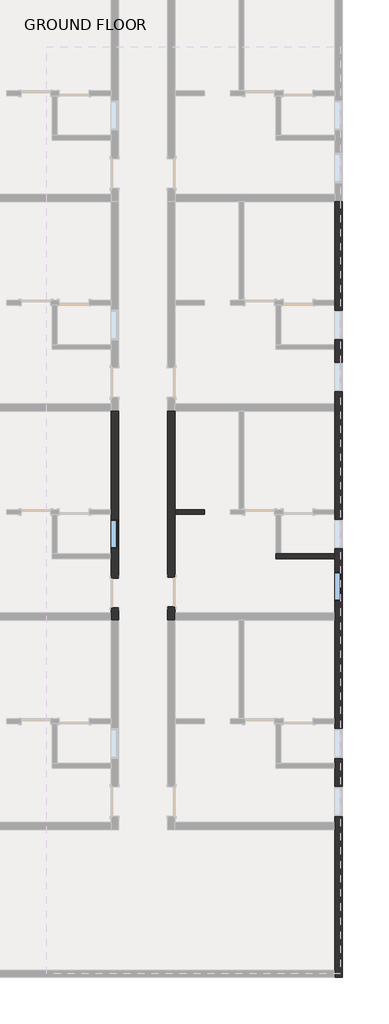
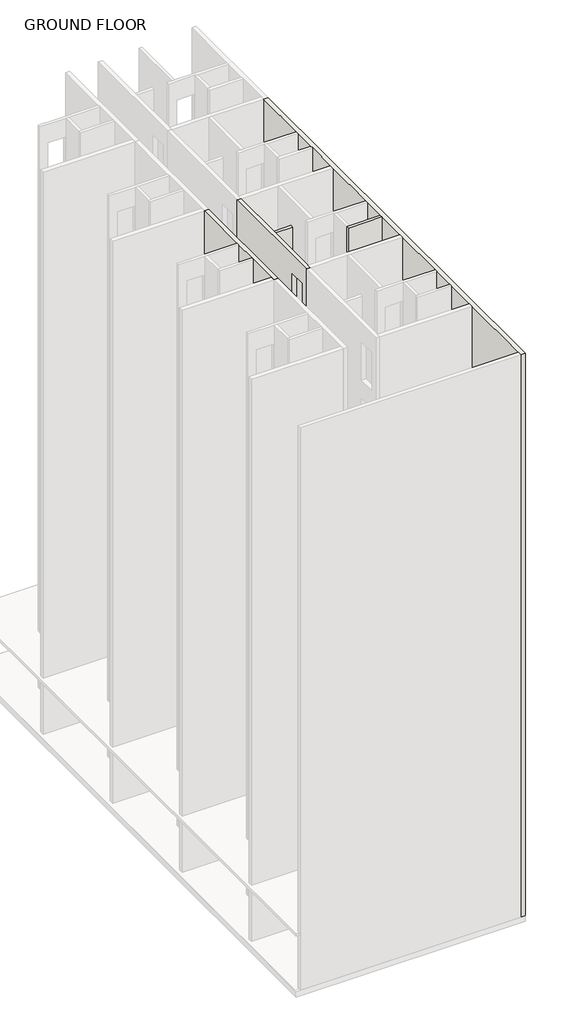
# One storey, part 4 of 7: 5 walls, 2 windows.
"""IFC4 building model written with IfcOpenShell, lengths in millimetres."""

from ifc_helpers import new_model, si_unit, origin, origin_with_axes, place, context, project, spatial, polyline, outline, extrude, faceted_brep, transform, mapped, element, save
from components import window_c1f32544

model = new_model("IFC4")

# Units and contexts
model_context = context("Model", 3, world=origin())
ifc_project = project(units=[si_unit("LENGTHUNIT", "METRE", prefix="MILLI")], contexts=[model_context])

# Site, building, storey
site = spatial("IfcSite", under=ifc_project)
building = spatial("IfcBuilding", under=site)
storey = spatial("IfcBuildingStorey", under=building, Name="GROUND FLOOR", Elevation=0.0)

# Walls
placement = place(None, origin())
element("IfcWall", 1, ObjectType="Generic - 8\"", at=placement, inside=storey, context=model_context, shape_type="Brep", body=[
    faceted_brep([(-5558.2902461, -4354.5289408, 0.0), (-5558.2902461, -4125.9289408, 0.0), (-5558.2902461, -3935.4289408, 0.0), (-5558.2902461, -3935.4289408, 2133.6), (-5558.2902461, -3021.0289408, 2133.6), (-5558.2902461, -3021.0289408, 0.0), (-5558.2902461, -1077.9289408, 0.0), (-5558.2902461, -925.5289408, 0.0), (-5558.2902461, 2122.4710592, 0.0), (-5558.2902461, 2122.4710592, 32004.0), (-5558.2902461, -925.5289408, 32004.0), (-5558.2902461, -1077.9289408, 32004.0), (-5558.2902461, -4125.9289408, 32004.0), (-5558.2902461, -4354.5289408, 32004.0), (-5558.2902461, -3021.0289408, 3200.4), (-5558.2902461, -3935.4289408, 3200.4), (-5558.2902461, -3935.4289408, 5334.0), (-5558.2902461, -3021.0289408, 5334.0), (-5558.2902461, -3021.0289408, 6400.8), (-5558.2902461, -3935.4289408, 6400.8), (-5558.2902461, -3935.4289408, 8534.4), (-5558.2902461, -3021.0289408, 8534.4), (-5558.2902461, -3021.0289408, 9601.2), (-5558.2902461, -3935.4289408, 9601.2), (-5558.2902461, -3935.4289408, 11734.8), (-5558.2902461, -3021.0289408, 11734.8), (-5558.2902461, -3021.0289408, 12801.6), (-5558.2902461, -3935.4289408, 12801.6), (-5558.2902461, -3935.4289408, 14935.2), (-5558.2902461, -3021.0289408, 14935.2), (-5558.2902461, -3021.0289408, 16002.0), (-5558.2902461, -3935.4289408, 16002.0), (-5558.2902461, -3935.4289408, 18135.6), (-5558.2902461, -3021.0289408, 18135.6), (-5558.2902461, -3021.0289408, 19202.4), (-5558.2902461, -3935.4289408, 19202.4), (-5558.2902461, -3935.4289408, 21336.0), (-5558.2902461, -3021.0289408, 21336.0), (-5558.2902461, -3021.0289408, 22402.8), (-5558.2902461, -3935.4289408, 22402.8), (-5558.2902461, -3935.4289408, 24536.4), (-5558.2902461, -3021.0289408, 24536.4), (-5558.2902461, -3021.0289408, 25603.2), (-5558.2902461, -3935.4289408, 25603.2), (-5558.2902461, -3935.4289408, 27736.8), (-5558.2902461, -3021.0289408, 27736.8), (-5558.2902461, -3021.0289408, 28803.6), (-5558.2902461, -3935.4289408, 28803.6), (-5558.2902461, -3935.4289408, 30937.2), (-5558.2902461, -3021.0289408, 30937.2), (-5786.8902461, -3935.4289408, 2133.6), (-5786.8902461, -3935.4289408, 0.0), (-5786.8902461, -4354.5289408, 0.0), (-5786.8902461, -4354.5289408, 32004.0), (-5786.8902461, 2122.4710592, 32004.0), (-5786.8902461, 2122.4710592, 0.0), (-5786.8902461, -3021.0289408, 0.0), (-5786.8902461, -3021.0289408, 2133.6), (-5786.8902461, -3021.0289408, 3200.4), (-5786.8902461, -3021.0289408, 5334.0), (-5786.8902461, -3935.4289408, 5334.0), (-5786.8902461, -3935.4289408, 3200.4), (-5786.8902461, -3021.0289408, 6400.8), (-5786.8902461, -3021.0289408, 8534.4), (-5786.8902461, -3935.4289408, 8534.4), (-5786.8902461, -3935.4289408, 6400.8), (-5786.8902461, -3021.0289408, 9601.2), (-5786.8902461, -3021.0289408, 11734.8), (-5786.8902461, -3935.4289408, 11734.8), (-5786.8902461, -3935.4289408, 9601.2), (-5786.8902461, -3021.0289408, 12801.6), (-5786.8902461, -3021.0289408, 14935.2), (-5786.8902461, -3935.4289408, 14935.2), (-5786.8902461, -3935.4289408, 12801.6), (-5786.8902461, -3021.0289408, 16002.0), (-5786.8902461, -3021.0289408, 18135.6), (-5786.8902461, -3935.4289408, 18135.6), (-5786.8902461, -3935.4289408, 16002.0), (-5786.8902461, -3021.0289408, 19202.4), (-5786.8902461, -3021.0289408, 21336.0), (-5786.8902461, -3935.4289408, 21336.0), (-5786.8902461, -3935.4289408, 19202.4), (-5786.8902461, -3021.0289408, 22402.8), (-5786.8902461, -3021.0289408, 24536.4), (-5786.8902461, -3935.4289408, 24536.4), (-5786.8902461, -3935.4289408, 22402.8), (-5786.8902461, -3021.0289408, 25603.2), (-5786.8902461, -3021.0289408, 27736.8), (-5786.8902461, -3935.4289408, 27736.8), (-5786.8902461, -3935.4289408, 25603.2), (-5786.8902461, -3021.0289408, 28803.6), (-5786.8902461, -3021.0289408, 30937.2), (-5786.8902461, -3935.4289408, 30937.2), (-5786.8902461, -3935.4289408, 28803.6)], [[[0, 1, 2, 3, 4, 5, 6, 7, 8, 9, 10, 11, 12, 13], [14, 15, 16, 17], [18, 19, 20, 21], [22, 23, 24, 25], [26, 27, 28, 29], [30, 31, 32, 33], [34, 35, 36, 37], [38, 39, 40, 41], [42, 43, 44, 45], [46, 47, 48, 49]], [[50, 51, 52, 53, 54, 55, 56, 57], [58, 59, 60, 61], [62, 63, 64, 65], [66, 67, 68, 69], [70, 71, 72, 73], [74, 75, 76, 77], [78, 79, 80, 81], [82, 83, 84, 85], [86, 87, 88, 89], [90, 91, 92, 93]], [[56, 55, 8, 7, 6, 5]], [[52, 51, 2, 1, 0]], [[13, 12, 11, 10, 9, 54, 53]], [[0, 13, 53, 52]], [[9, 8, 55, 54]], [[3, 2, 51, 50]], [[4, 3, 50, 57]], [[5, 4, 57, 56]], [[15, 14, 58, 61]], [[16, 15, 61, 60]], [[17, 16, 60, 59]], [[14, 17, 59, 58]], [[19, 18, 62, 65]], [[20, 19, 65, 64]], [[21, 20, 64, 63]], [[18, 21, 63, 62]], [[23, 22, 66, 69]], [[24, 23, 69, 68]], [[25, 24, 68, 67]], [[22, 25, 67, 66]], [[27, 26, 70, 73]], [[28, 27, 73, 72]], [[29, 28, 72, 71]], [[26, 29, 71, 70]], [[31, 30, 74, 77]], [[32, 31, 77, 76]], [[33, 32, 76, 75]], [[30, 33, 75, 74]], [[35, 34, 78, 81]], [[36, 35, 81, 80]], [[37, 36, 80, 79]], [[34, 37, 79, 78]], [[39, 38, 82, 85]], [[40, 39, 85, 84]], [[41, 40, 84, 83]], [[38, 41, 83, 82]], [[43, 42, 86, 89]], [[44, 43, 89, 88]], [[45, 44, 88, 87]], [[42, 45, 87, 86]], [[47, 46, 90, 93]], [[48, 47, 93, 92]], [[49, 48, 92, 91]], [[46, 49, 91, 90]]]),
])
element("IfcWall", 2, ObjectType="INNER WALL 2", at=placement, inside=storey, context=model_context, shape_type="Brep", body=[
    faceted_brep([(-605.2902461, -2297.1289408, 0.0), (-2281.6902461, -2297.1289408, 0.0), (-2434.0902461, -2297.1289408, 0.0), (-2434.0902461, -2297.1289408, 32004.0), (-2281.6902461, -2297.1289408, 32004.0), (-605.2902461, -2297.1289408, 32004.0), (-605.2902461, -2449.5289408, 0.0), (-605.2902461, -2449.5289408, 32004.0), (-2434.0902461, -2449.5289408, 32004.0), (-2434.0902461, -2449.5289408, 0.0)], [[[0, 1, 2, 3, 4, 5]], [[6, 7, 8, 9]], [[2, 1, 0, 6, 9]], [[5, 4, 3, 8, 7]], [[3, 2, 9, 8]], [[0, 5, 7, 6]]]),
])
element("IfcWall", 3, ObjectType="INNER WALL 2", at=placement, inside=storey, context=model_context, shape_type="SweptSolid", body=[
    extrude(outline(polyline([(-4643.8902461, -1077.9289408), (-5558.2902461, -1077.9289408), (-5558.2902461, -925.5289408), (-4643.8902461, -925.5289408), (-4643.8902461, -1077.9289408)])), origin_with_axes(), (0.0, 0.0, 1.0), 32004.0),
])
element("IfcWall", 4, ObjectType="OUTER WALL", at=placement, inside=storey, context=model_context, shape_type="Brep", body=[
    faceted_brep([(-376.6902461, -15403.5289408, 0.0), (-376.6902461, 8599.4710592, 0.0), (-376.6902461, 8599.4710592, 32004.0), (-376.6902461, -15403.5289408, 32004.0), (-376.6902461, -10412.4289408, 2133.6), (-376.6902461, -9498.0289408, 2133.6), (-376.6902461, -9498.0289408, 914.4), (-376.6902461, -10412.4289408, 914.4), (-376.6902461, -8621.7289408, 2133.6), (-376.6902461, -7707.3289408, 2133.6), (-376.6902461, -7707.3289408, 914.4), (-376.6902461, -8621.7289408, 914.4), (-376.6902461, -3763.9789408, 2133.6), (-376.6902461, -2849.5789408, 2133.6), (-376.6902461, -2849.5789408, 914.4), (-376.6902461, -3763.9789408, 914.4), (-376.6902461, -2144.7289408, 2133.6), (-376.6902461, -1230.3289408, 2133.6), (-376.6902461, -1230.3289408, 914.4), (-376.6902461, -2144.7289408, 914.4), (-376.6902461, 2713.0210592, 2133.6), (-376.6902461, 3627.4210592, 2133.6), (-376.6902461, 3627.4210592, 914.4), (-376.6902461, 2713.0210592, 914.4), (-376.6902461, 4332.2710592, 2133.6), (-376.6902461, 5246.6710592, 2133.6), (-376.6902461, 5246.6710592, 914.4), (-376.6902461, 4332.2710592, 914.4), (-376.6902461, 4332.2710592, 5334.0), (-376.6902461, 5246.6710592, 5334.0), (-376.6902461, 5246.6710592, 4114.8), (-376.6902461, 4332.2710592, 4114.8), (-376.6902461, 2713.0210592, 5334.0), (-376.6902461, 3627.4210592, 5334.0), (-376.6902461, 3627.4210592, 4114.8), (-376.6902461, 2713.0210592, 4114.8), (-376.6902461, -2144.7289408, 5334.0), (-376.6902461, -1230.3289408, 5334.0), (-376.6902461, -1230.3289408, 4114.8), (-376.6902461, -2144.7289408, 4114.8), (-376.6902461, -3763.9789408, 5334.0), (-376.6902461, -2849.5789408, 5334.0), (-376.6902461, -2849.5789408, 4114.8), (-376.6902461, -3763.9789408, 4114.8), (-376.6902461, -8621.7289408, 5334.0), (-376.6902461, -7707.3289408, 5334.0), (-376.6902461, -7707.3289408, 4114.8), (-376.6902461, -8621.7289408, 4114.8), (-376.6902461, -10412.4289408, 5334.0), (-376.6902461, -9498.0289408, 5334.0), (-376.6902461, -9498.0289408, 4114.8), (-376.6902461, -10412.4289408, 4114.8), (-376.6902461, 4332.2710592, 8534.4), (-376.6902461, 5246.6710592, 8534.4), (-376.6902461, 5246.6710592, 7315.2), (-376.6902461, 4332.2710592, 7315.2), (-376.6902461, 2713.0210592, 8534.4), (-376.6902461, 3627.4210592, 8534.4), (-376.6902461, 3627.4210592, 7315.2), (-376.6902461, 2713.0210592, 7315.2), (-376.6902461, -2144.7289408, 8534.4), (-376.6902461, -1230.3289408, 8534.4), (-376.6902461, -1230.3289408, 7315.2), (-376.6902461, -2144.7289408, 7315.2), (-376.6902461, -3763.9789408, 8534.4), (-376.6902461, -2849.5789408, 8534.4), (-376.6902461, -2849.5789408, 7315.2), (-376.6902461, -3763.9789408, 7315.2), (-376.6902461, -8621.7289408, 8534.4), (-376.6902461, -7707.3289408, 8534.4), (-376.6902461, -7707.3289408, 7315.2), (-376.6902461, -8621.7289408, 7315.2), (-376.6902461, -10412.4289408, 8534.4), (-376.6902461, -9498.0289408, 8534.4), (-376.6902461, -9498.0289408, 7315.2), (-376.6902461, -10412.4289408, 7315.2), (-376.6902461, 4332.2710592, 11734.8), (-376.6902461, 5246.6710592, 11734.8), (-376.6902461, 5246.6710592, 10515.6), (-376.6902461, 4332.2710592, 10515.6), (-376.6902461, 2713.0210592, 11734.8), (-376.6902461, 3627.4210592, 11734.8), (-376.6902461, 3627.4210592, 10515.6), (-376.6902461, 2713.0210592, 10515.6), (-376.6902461, -2144.7289408, 11734.8), (-376.6902461, -1230.3289408, 11734.8), (-376.6902461, -1230.3289408, 10515.6), (-376.6902461, -2144.7289408, 10515.6), (-376.6902461, -3763.9789408, 11734.8), (-376.6902461, -2849.5789408, 11734.8), (-376.6902461, -2849.5789408, 10515.6), (-376.6902461, -3763.9789408, 10515.6), (-376.6902461, -8621.7289408, 11734.8), (-376.6902461, -7707.3289408, 11734.8), (-376.6902461, -7707.3289408, 10515.6), (-376.6902461, -8621.7289408, 10515.6), (-376.6902461, -10412.4289408, 11734.8), (-376.6902461, -9498.0289408, 11734.8), (-376.6902461, -9498.0289408, 10515.6), (-376.6902461, -10412.4289408, 10515.6), (-376.6902461, 4332.2710592, 14935.2), (-376.6902461, 5246.6710592, 14935.2), (-376.6902461, 5246.6710592, 13716.0), (-376.6902461, 4332.2710592, 13716.0), (-376.6902461, 2713.0210592, 14935.2), (-376.6902461, 3627.4210592, 14935.2), (-376.6902461, 3627.4210592, 13716.0), (-376.6902461, 2713.0210592, 13716.0), (-376.6902461, -2144.7289408, 14935.2), (-376.6902461, -1230.3289408, 14935.2), (-376.6902461, -1230.3289408, 13716.0), (-376.6902461, -2144.7289408, 13716.0), (-376.6902461, -3763.9789408, 14935.2), (-376.6902461, -2849.5789408, 14935.2), (-376.6902461, -2849.5789408, 13716.0), (-376.6902461, -3763.9789408, 13716.0), (-376.6902461, -8621.7289408, 14935.2), (-376.6902461, -7707.3289408, 14935.2), (-376.6902461, -7707.3289408, 13716.0), (-376.6902461, -8621.7289408, 13716.0), (-376.6902461, -10412.4289408, 14935.2), (-376.6902461, -9498.0289408, 14935.2), (-376.6902461, -9498.0289408, 13716.0), (-376.6902461, -10412.4289408, 13716.0), (-376.6902461, 4332.2710592, 18135.6), (-376.6902461, 5246.6710592, 18135.6), (-376.6902461, 5246.6710592, 16916.4), (-376.6902461, 4332.2710592, 16916.4), (-376.6902461, 2713.0210592, 18135.6), (-376.6902461, 3627.4210592, 18135.6), (-376.6902461, 3627.4210592, 16916.4), (-376.6902461, 2713.0210592, 16916.4), (-376.6902461, -2144.7289408, 18135.6), (-376.6902461, -1230.3289408, 18135.6), (-376.6902461, -1230.3289408, 16916.4), (-376.6902461, -2144.7289408, 16916.4), (-376.6902461, -3763.9789408, 18135.6), (-376.6902461, -2849.5789408, 18135.6), (-376.6902461, -2849.5789408, 16916.4), (-376.6902461, -3763.9789408, 16916.4), (-376.6902461, -8621.7289408, 18135.6), (-376.6902461, -7707.3289408, 18135.6), (-376.6902461, -7707.3289408, 16916.4), (-376.6902461, -8621.7289408, 16916.4), (-376.6902461, -10412.4289408, 18135.6), (-376.6902461, -9498.0289408, 18135.6), (-376.6902461, -9498.0289408, 16916.4), (-376.6902461, -10412.4289408, 16916.4), (-376.6902461, 4332.2710592, 21336.0), (-376.6902461, 5246.6710592, 21336.0), (-376.6902461, 5246.6710592, 20116.8), (-376.6902461, 4332.2710592, 20116.8), (-376.6902461, 2713.0210592, 21336.0), (-376.6902461, 3627.4210592, 21336.0), (-376.6902461, 3627.4210592, 20116.8), (-376.6902461, 2713.0210592, 20116.8), (-376.6902461, -2144.7289408, 21336.0), (-376.6902461, -1230.3289408, 21336.0), (-376.6902461, -1230.3289408, 20116.8), (-376.6902461, -2144.7289408, 20116.8), (-376.6902461, -3763.9789408, 21336.0), (-376.6902461, -2849.5789408, 21336.0), (-376.6902461, -2849.5789408, 20116.8), (-376.6902461, -3763.9789408, 20116.8), (-376.6902461, -8621.7289408, 21336.0), (-376.6902461, -7707.3289408, 21336.0), (-376.6902461, -7707.3289408, 20116.8), (-376.6902461, -8621.7289408, 20116.8), (-376.6902461, -10412.4289408, 21336.0), (-376.6902461, -9498.0289408, 21336.0), (-376.6902461, -9498.0289408, 20116.8), (-376.6902461, -10412.4289408, 20116.8), (-376.6902461, 4332.2710592, 24536.4), (-376.6902461, 5246.6710592, 24536.4), (-376.6902461, 5246.6710592, 23317.2), (-376.6902461, 4332.2710592, 23317.2), (-376.6902461, 2713.0210592, 24536.4), (-376.6902461, 3627.4210592, 24536.4), (-376.6902461, 3627.4210592, 23317.2), (-376.6902461, 2713.0210592, 23317.2), (-376.6902461, -2144.7289408, 24536.4), (-376.6902461, -1230.3289408, 24536.4), (-376.6902461, -1230.3289408, 23317.2), (-376.6902461, -2144.7289408, 23317.2), (-376.6902461, -3763.9789408, 24536.4), (-376.6902461, -2849.5789408, 24536.4), (-376.6902461, -2849.5789408, 23317.2), (-376.6902461, -3763.9789408, 23317.2), (-376.6902461, -8621.7289408, 24536.4), (-376.6902461, -7707.3289408, 24536.4), (-376.6902461, -7707.3289408, 23317.2), (-376.6902461, -8621.7289408, 23317.2), (-376.6902461, -10412.4289408, 24536.4), (-376.6902461, -9498.0289408, 24536.4), (-376.6902461, -9498.0289408, 23317.2), (-376.6902461, -10412.4289408, 23317.2), (-376.6902461, 4332.2710592, 27736.8), (-376.6902461, 5246.6710592, 27736.8), (-376.6902461, 5246.6710592, 26517.6), (-376.6902461, 4332.2710592, 26517.6), (-376.6902461, -2144.7289408, 27736.8), (-376.6902461, -1230.3289408, 27736.8), (-376.6902461, -1230.3289408, 26517.6), (-376.6902461, -2144.7289408, 26517.6), (-376.6902461, -8621.7289408, 27736.8), (-376.6902461, -7707.3289408, 27736.8), (-376.6902461, -7707.3289408, 26517.6), (-376.6902461, -8621.7289408, 26517.6), (-376.6902461, -10412.4289408, 27736.8), (-376.6902461, -9498.0289408, 27736.8), (-376.6902461, -9498.0289408, 26517.6), (-376.6902461, -10412.4289408, 26517.6), (-376.6902461, -3763.9789408, 27736.8), (-376.6902461, -2849.5789408, 27736.8), (-376.6902461, -2849.5789408, 26517.6), (-376.6902461, -3763.9789408, 26517.6), (-376.6902461, 2713.0210592, 27736.8), (-376.6902461, 3627.4210592, 27736.8), (-376.6902461, 3627.4210592, 26517.6), (-376.6902461, 2713.0210592, 26517.6), (-376.6902461, 4332.2710592, 30937.2), (-376.6902461, 5246.6710592, 30937.2), (-376.6902461, 5246.6710592, 29718.0), (-376.6902461, 4332.2710592, 29718.0), (-376.6902461, 2713.0210592, 30937.2), (-376.6902461, 3627.4210592, 30937.2), (-376.6902461, 3627.4210592, 29718.0), (-376.6902461, 2713.0210592, 29718.0), (-376.6902461, -2144.7289408, 30937.2), (-376.6902461, -1230.3289408, 30937.2), (-376.6902461, -1230.3289408, 29718.0), (-376.6902461, -2144.7289408, 29718.0), (-376.6902461, -3763.9789408, 30937.2), (-376.6902461, -2849.5789408, 30937.2), (-376.6902461, -2849.5789408, 29718.0), (-376.6902461, -3763.9789408, 29718.0), (-376.6902461, -8621.7289408, 30937.2), (-376.6902461, -7707.3289408, 30937.2), (-376.6902461, -7707.3289408, 29718.0), (-376.6902461, -8621.7289408, 29718.0), (-376.6902461, -10412.4289408, 30937.2), (-376.6902461, -9498.0289408, 30937.2), (-376.6902461, -9498.0289408, 29718.0), (-376.6902461, -10412.4289408, 29718.0), (-605.2902461, -15403.5289408, 0.0), (-605.2902461, -15403.5289408, 32004.0), (-605.2902461, -15174.9289408, 32004.0), (-605.2902461, -10831.5289408, 32004.0), (-605.2902461, -10602.9289408, 32004.0), (-605.2902461, -8926.5289408, 32004.0), (-605.2902461, -8774.1289408, 32004.0), (-605.2902461, -7554.9289408, 32004.0), (-605.2902461, -7402.5289408, 32004.0), (-605.2902461, -4354.5289408, 32004.0), (-605.2902461, -4125.9289408, 32004.0), (-605.2902461, -2449.5289408, 32004.0), (-605.2902461, -2297.1289408, 32004.0), (-605.2902461, -1077.9289408, 32004.0), (-605.2902461, -925.5289408, 32004.0), (-605.2902461, 2122.4710592, 32004.0), (-605.2902461, 2351.0710592, 32004.0), (-605.2902461, 4027.4710592, 32004.0), (-605.2902461, 4179.8710592, 32004.0), (-605.2902461, 5399.0710592, 32004.0), (-605.2902461, 5551.4710592, 32004.0), (-605.2902461, 8599.4710592, 32004.0), (-605.2902461, 8599.4710592, 0.0), (-605.2902461, 5551.4710592, 0.0), (-605.2902461, 5399.0710592, 0.0), (-605.2902461, 4179.8710592, 0.0), (-605.2902461, 4027.4710592, 0.0), (-605.2902461, 2351.0710592, 0.0), (-605.2902461, 2122.4710592, 0.0), (-605.2902461, -925.5289408, 0.0), (-605.2902461, -1077.9289408, 0.0), (-605.2902461, -2297.1289408, 0.0), (-605.2902461, -2449.5289408, 0.0), (-605.2902461, -4125.9289408, 0.0), (-605.2902461, -4354.5289408, 0.0), (-605.2902461, -7402.5289408, 0.0), (-605.2902461, -7554.9289408, 0.0), (-605.2902461, -8774.1289408, 0.0), (-605.2902461, -8926.5289408, 0.0), (-605.2902461, -10602.9289408, 0.0), (-605.2902461, -10831.5289408, 0.0), (-605.2902461, -15174.9289408, 0.0), (-605.2902461, -10412.4289408, 2133.6), (-605.2902461, -10412.4289408, 914.4), (-605.2902461, -9498.0289408, 914.4), (-605.2902461, -9498.0289408, 2133.6), (-605.2902461, -8621.7289408, 2133.6), (-605.2902461, -8621.7289408, 914.4), (-605.2902461, -7707.3289408, 914.4), (-605.2902461, -7707.3289408, 2133.6), (-605.2902461, -3763.9789408, 2133.6), (-605.2902461, -3763.9789408, 914.4), (-605.2902461, -2849.5789408, 914.4), (-605.2902461, -2849.5789408, 2133.6), (-605.2902461, -2144.7289408, 2133.6), (-605.2902461, -2144.7289408, 914.4), (-605.2902461, -1230.3289408, 914.4), (-605.2902461, -1230.3289408, 2133.6), (-605.2902461, 2713.0210592, 2133.6), (-605.2902461, 2713.0210592, 914.4), (-605.2902461, 3627.4210592, 914.4), (-605.2902461, 3627.4210592, 2133.6), (-605.2902461, 4332.2710592, 2133.6), (-605.2902461, 4332.2710592, 914.4), (-605.2902461, 5246.6710592, 914.4), (-605.2902461, 5246.6710592, 2133.6), (-605.2902461, 4332.2710592, 5334.0), (-605.2902461, 4332.2710592, 4114.8), (-605.2902461, 5246.6710592, 4114.8), (-605.2902461, 5246.6710592, 5334.0), (-605.2902461, 2713.0210592, 5334.0), (-605.2902461, 2713.0210592, 4114.8), (-605.2902461, 3627.4210592, 4114.8), (-605.2902461, 3627.4210592, 5334.0), (-605.2902461, -2144.7289408, 5334.0), (-605.2902461, -2144.7289408, 4114.8), (-605.2902461, -1230.3289408, 4114.8), (-605.2902461, -1230.3289408, 5334.0), (-605.2902461, -3763.9789408, 5334.0), (-605.2902461, -3763.9789408, 4114.8), (-605.2902461, -2849.5789408, 4114.8), (-605.2902461, -2849.5789408, 5334.0), (-605.2902461, -8621.7289408, 5334.0), (-605.2902461, -8621.7289408, 4114.8), (-605.2902461, -7707.3289408, 4114.8), (-605.2902461, -7707.3289408, 5334.0), (-605.2902461, -10412.4289408, 5334.0), (-605.2902461, -10412.4289408, 4114.8), (-605.2902461, -9498.0289408, 4114.8), (-605.2902461, -9498.0289408, 5334.0), (-605.2902461, 4332.2710592, 8534.4), (-605.2902461, 4332.2710592, 7315.2), (-605.2902461, 5246.6710592, 7315.2), (-605.2902461, 5246.6710592, 8534.4), (-605.2902461, 2713.0210592, 8534.4), (-605.2902461, 2713.0210592, 7315.2), (-605.2902461, 3627.4210592, 7315.2), (-605.2902461, 3627.4210592, 8534.4), (-605.2902461, -2144.7289408, 8534.4), (-605.2902461, -2144.7289408, 7315.2), (-605.2902461, -1230.3289408, 7315.2), (-605.2902461, -1230.3289408, 8534.4), (-605.2902461, -3763.9789408, 8534.4), (-605.2902461, -3763.9789408, 7315.2), (-605.2902461, -2849.5789408, 7315.2), (-605.2902461, -2849.5789408, 8534.4), (-605.2902461, -8621.7289408, 8534.4), (-605.2902461, -8621.7289408, 7315.2), (-605.2902461, -7707.3289408, 7315.2), (-605.2902461, -7707.3289408, 8534.4), (-605.2902461, -10412.4289408, 8534.4), (-605.2902461, -10412.4289408, 7315.2), (-605.2902461, -9498.0289408, 7315.2), (-605.2902461, -9498.0289408, 8534.4), (-605.2902461, 4332.2710592, 11734.8), (-605.2902461, 4332.2710592, 10515.6), (-605.2902461, 5246.6710592, 10515.6), (-605.2902461, 5246.6710592, 11734.8), (-605.2902461, 2713.0210592, 11734.8), (-605.2902461, 2713.0210592, 10515.6), (-605.2902461, 3627.4210592, 10515.6), (-605.2902461, 3627.4210592, 11734.8), (-605.2902461, -2144.7289408, 11734.8), (-605.2902461, -2144.7289408, 10515.6), (-605.2902461, -1230.3289408, 10515.6), (-605.2902461, -1230.3289408, 11734.8), (-605.2902461, -3763.9789408, 11734.8), (-605.2902461, -3763.9789408, 10515.6), (-605.2902461, -2849.5789408, 10515.6), (-605.2902461, -2849.5789408, 11734.8), (-605.2902461, -8621.7289408, 11734.8), (-605.2902461, -8621.7289408, 10515.6), (-605.2902461, -7707.3289408, 10515.6), (-605.2902461, -7707.3289408, 11734.8), (-605.2902461, -10412.4289408, 11734.8), (-605.2902461, -10412.4289408, 10515.6), (-605.2902461, -9498.0289408, 10515.6), (-605.2902461, -9498.0289408, 11734.8), (-605.2902461, 4332.2710592, 14935.2), (-605.2902461, 4332.2710592, 13716.0), (-605.2902461, 5246.6710592, 13716.0), (-605.2902461, 5246.6710592, 14935.2), (-605.2902461, 2713.0210592, 14935.2), (-605.2902461, 2713.0210592, 13716.0), (-605.2902461, 3627.4210592, 13716.0), (-605.2902461, 3627.4210592, 14935.2), (-605.2902461, -2144.7289408, 14935.2), (-605.2902461, -2144.7289408, 13716.0), (-605.2902461, -1230.3289408, 13716.0), (-605.2902461, -1230.3289408, 14935.2), (-605.2902461, -3763.9789408, 14935.2), (-605.2902461, -3763.9789408, 13716.0), (-605.2902461, -2849.5789408, 13716.0), (-605.2902461, -2849.5789408, 14935.2), (-605.2902461, -8621.7289408, 14935.2), (-605.2902461, -8621.7289408, 13716.0), (-605.2902461, -7707.3289408, 13716.0), (-605.2902461, -7707.3289408, 14935.2), (-605.2902461, -10412.4289408, 14935.2), (-605.2902461, -10412.4289408, 13716.0), (-605.2902461, -9498.0289408, 13716.0), (-605.2902461, -9498.0289408, 14935.2), (-605.2902461, 4332.2710592, 18135.6), (-605.2902461, 4332.2710592, 16916.4), (-605.2902461, 5246.6710592, 16916.4), (-605.2902461, 5246.6710592, 18135.6), (-605.2902461, 2713.0210592, 18135.6), (-605.2902461, 2713.0210592, 16916.4), (-605.2902461, 3627.4210592, 16916.4), (-605.2902461, 3627.4210592, 18135.6), (-605.2902461, -2144.7289408, 18135.6), (-605.2902461, -2144.7289408, 16916.4), (-605.2902461, -1230.3289408, 16916.4), (-605.2902461, -1230.3289408, 18135.6), (-605.2902461, -3763.9789408, 18135.6), (-605.2902461, -3763.9789408, 16916.4), (-605.2902461, -2849.5789408, 16916.4), (-605.2902461, -2849.5789408, 18135.6), (-605.2902461, -8621.7289408, 18135.6), (-605.2902461, -8621.7289408, 16916.4), (-605.2902461, -7707.3289408, 16916.4), (-605.2902461, -7707.3289408, 18135.6), (-605.2902461, -10412.4289408, 18135.6), (-605.2902461, -10412.4289408, 16916.4), (-605.2902461, -9498.0289408, 16916.4), (-605.2902461, -9498.0289408, 18135.6), (-605.2902461, 4332.2710592, 21336.0), (-605.2902461, 4332.2710592, 20116.8), (-605.2902461, 5246.6710592, 20116.8), (-605.2902461, 5246.6710592, 21336.0), (-605.2902461, 2713.0210592, 21336.0), (-605.2902461, 2713.0210592, 20116.8), (-605.2902461, 3627.4210592, 20116.8), (-605.2902461, 3627.4210592, 21336.0), (-605.2902461, -2144.7289408, 21336.0), (-605.2902461, -2144.7289408, 20116.8), (-605.2902461, -1230.3289408, 20116.8), (-605.2902461, -1230.3289408, 21336.0), (-605.2902461, -3763.9789408, 21336.0), (-605.2902461, -3763.9789408, 20116.8), (-605.2902461, -2849.5789408, 20116.8), (-605.2902461, -2849.5789408, 21336.0), (-605.2902461, -8621.7289408, 21336.0), (-605.2902461, -8621.7289408, 20116.8), (-605.2902461, -7707.3289408, 20116.8), (-605.2902461, -7707.3289408, 21336.0), (-605.2902461, -10412.4289408, 21336.0), (-605.2902461, -10412.4289408, 20116.8), (-605.2902461, -9498.0289408, 20116.8), (-605.2902461, -9498.0289408, 21336.0), (-605.2902461, 4332.2710592, 24536.4), (-605.2902461, 4332.2710592, 23317.2), (-605.2902461, 5246.6710592, 23317.2), (-605.2902461, 5246.6710592, 24536.4), (-605.2902461, 2713.0210592, 24536.4), (-605.2902461, 2713.0210592, 23317.2), (-605.2902461, 3627.4210592, 23317.2), (-605.2902461, 3627.4210592, 24536.4), (-605.2902461, -2144.7289408, 24536.4), (-605.2902461, -2144.7289408, 23317.2), (-605.2902461, -1230.3289408, 23317.2), (-605.2902461, -1230.3289408, 24536.4), (-605.2902461, -3763.9789408, 24536.4), (-605.2902461, -3763.9789408, 23317.2), (-605.2902461, -2849.5789408, 23317.2), (-605.2902461, -2849.5789408, 24536.4), (-605.2902461, -8621.7289408, 24536.4), (-605.2902461, -8621.7289408, 23317.2), (-605.2902461, -7707.3289408, 23317.2), (-605.2902461, -7707.3289408, 24536.4), (-605.2902461, -10412.4289408, 24536.4), (-605.2902461, -10412.4289408, 23317.2), (-605.2902461, -9498.0289408, 23317.2), (-605.2902461, -9498.0289408, 24536.4), (-605.2902461, 4332.2710592, 27736.8), (-605.2902461, 4332.2710592, 26517.6), (-605.2902461, 5246.6710592, 26517.6), (-605.2902461, 5246.6710592, 27736.8), (-605.2902461, -2144.7289408, 27736.8), (-605.2902461, -2144.7289408, 26517.6), (-605.2902461, -1230.3289408, 26517.6), (-605.2902461, -1230.3289408, 27736.8), (-605.2902461, -8621.7289408, 27736.8), (-605.2902461, -8621.7289408, 26517.6), (-605.2902461, -7707.3289408, 26517.6), (-605.2902461, -7707.3289408, 27736.8), (-605.2902461, -10412.4289408, 27736.8), (-605.2902461, -10412.4289408, 26517.6), (-605.2902461, -9498.0289408, 26517.6), (-605.2902461, -9498.0289408, 27736.8), (-605.2902461, -3763.9789408, 27736.8), (-605.2902461, -3763.9789408, 26517.6), (-605.2902461, -2849.5789408, 26517.6), (-605.2902461, -2849.5789408, 27736.8), (-605.2902461, 2713.0210592, 27736.8), (-605.2902461, 2713.0210592, 26517.6), (-605.2902461, 3627.4210592, 26517.6), (-605.2902461, 3627.4210592, 27736.8), (-605.2902461, 4332.2710592, 30937.2), (-605.2902461, 4332.2710592, 29718.0), (-605.2902461, 5246.6710592, 29718.0), (-605.2902461, 5246.6710592, 30937.2), (-605.2902461, 2713.0210592, 30937.2), (-605.2902461, 2713.0210592, 29718.0), (-605.2902461, 3627.4210592, 29718.0), (-605.2902461, 3627.4210592, 30937.2), (-605.2902461, -2144.7289408, 30937.2), (-605.2902461, -2144.7289408, 29718.0), (-605.2902461, -1230.3289408, 29718.0), (-605.2902461, -1230.3289408, 30937.2), (-605.2902461, -3763.9789408, 30937.2), (-605.2902461, -3763.9789408, 29718.0), (-605.2902461, -2849.5789408, 29718.0), (-605.2902461, -2849.5789408, 30937.2), (-605.2902461, -8621.7289408, 30937.2), (-605.2902461, -8621.7289408, 29718.0), (-605.2902461, -7707.3289408, 29718.0), (-605.2902461, -7707.3289408, 30937.2), (-605.2902461, -10412.4289408, 30937.2), (-605.2902461, -10412.4289408, 29718.0), (-605.2902461, -9498.0289408, 29718.0), (-605.2902461, -9498.0289408, 30937.2)], [[[0, 1, 2, 3], [4, 5, 6, 7], [8, 9, 10, 11], [12, 13, 14, 15], [16, 17, 18, 19], [20, 21, 22, 23], [24, 25, 26, 27], [28, 29, 30, 31], [32, 33, 34, 35], [36, 37, 38, 39], [40, 41, 42, 43], [44, 45, 46, 47], [48, 49, 50, 51], [52, 53, 54, 55], [56, 57, 58, 59], [60, 61, 62, 63], [64, 65, 66, 67], [68, 69, 70, 71], [72, 73, 74, 75], [76, 77, 78, 79], [80, 81, 82, 83], [84, 85, 86, 87], [88, 89, 90, 91], [92, 93, 94, 95], [96, 97, 98, 99], [100, 101, 102, 103], [104, 105, 106, 107], [108, 109, 110, 111], [112, 113, 114, 115], [116, 117, 118, 119], [120, 121, 122, 123], [124, 125, 126, 127], [128, 129, 130, 131], [132, 133, 134, 135], [136, 137, 138, 139], [140, 141, 142, 143], [144, 145, 146, 147], [148, 149, 150, 151], [152, 153, 154, 155], [156, 157, 158, 159], [160, 161, 162, 163], [164, 165, 166, 167], [168, 169, 170, 171], [172, 173, 174, 175], [176, 177, 178, 179], [180, 181, 182, 183], [184, 185, 186, 187], [188, 189, 190, 191], [192, 193, 194, 195], [196, 197, 198, 199], [200, 201, 202, 203], [204, 205, 206, 207], [208, 209, 210, 211], [212, 213, 214, 215], [216, 217, 218, 219], [220, 221, 222, 223], [224, 225, 226, 227], [228, 229, 230, 231], [232, 233, 234, 235], [236, 237, 238, 239], [240, 241, 242, 243]], [[244, 245, 246, 247, 248, 249, 250, 251, 252, 253, 254, 255, 256, 257, 258, 259, 260, 261, 262, 263, 264, 265, 266, 267, 268, 269, 270, 271, 272, 273, 274, 275, 276, 277, 278, 279, 280, 281, 282, 283, 284, 285], [286, 287, 288, 289], [290, 291, 292, 293], [294, 295, 296, 297], [298, 299, 300, 301], [302, 303, 304, 305], [306, 307, 308, 309], [310, 311, 312, 313], [314, 315, 316, 317], [318, 319, 320, 321], [322, 323, 324, 325], [326, 327, 328, 329], [330, 331, 332, 333], [334, 335, 336, 337], [338, 339, 340, 341], [342, 343, 344, 345], [346, 347, 348, 349], [350, 351, 352, 353], [354, 355, 356, 357], [358, 359, 360, 361], [362, 363, 364, 365], [366, 367, 368, 369], [370, 371, 372, 373], [374, 375, 376, 377], [378, 379, 380, 381], [382, 383, 384, 385], [386, 387, 388, 389], [390, 391, 392, 393], [394, 395, 396, 397], [398, 399, 400, 401], [402, 403, 404, 405], [406, 407, 408, 409], [410, 411, 412, 413], [414, 415, 416, 417], [418, 419, 420, 421], [422, 423, 424, 425], [426, 427, 428, 429], [430, 431, 432, 433], [434, 435, 436, 437], [438, 439, 440, 441], [442, 443, 444, 445], [446, 447, 448, 449], [450, 451, 452, 453], [454, 455, 456, 457], [458, 459, 460, 461], [462, 463, 464, 465], [466, 467, 468, 469], [470, 471, 472, 473], [474, 475, 476, 477], [478, 479, 480, 481], [482, 483, 484, 485], [486, 487, 488, 489], [490, 491, 492, 493], [494, 495, 496, 497], [498, 499, 500, 501], [502, 503, 504, 505], [506, 507, 508, 509], [510, 511, 512, 513], [514, 515, 516, 517], [518, 519, 520, 521], [522, 523, 524, 525]], [[1, 0, 244, 285, 284, 283, 282, 281, 280, 279, 278, 277, 276, 275, 274, 273, 272, 271, 270, 269, 268, 267, 266]], [[3, 2, 265, 264, 263, 262, 261, 260, 259, 258, 257, 256, 255, 254, 253, 252, 251, 250, 249, 248, 247, 246, 245]], [[2, 1, 266, 265]], [[287, 286, 4, 7]], [[288, 287, 7, 6]], [[289, 288, 6, 5]], [[286, 289, 5, 4]], [[291, 290, 8, 11]], [[292, 291, 11, 10]], [[293, 292, 10, 9]], [[290, 293, 9, 8]], [[295, 294, 12, 15]], [[296, 295, 15, 14]], [[297, 296, 14, 13]], [[294, 297, 13, 12]], [[299, 298, 16, 19]], [[300, 299, 19, 18]], [[301, 300, 18, 17]], [[298, 301, 17, 16]], [[303, 302, 20, 23]], [[304, 303, 23, 22]], [[305, 304, 22, 21]], [[302, 305, 21, 20]], [[307, 306, 24, 27]], [[308, 307, 27, 26]], [[309, 308, 26, 25]], [[306, 309, 25, 24]], [[311, 310, 28, 31]], [[312, 311, 31, 30]], [[313, 312, 30, 29]], [[310, 313, 29, 28]], [[315, 314, 32, 35]], [[316, 315, 35, 34]], [[317, 316, 34, 33]], [[314, 317, 33, 32]], [[319, 318, 36, 39]], [[320, 319, 39, 38]], [[321, 320, 38, 37]], [[318, 321, 37, 36]], [[323, 322, 40, 43]], [[324, 323, 43, 42]], [[325, 324, 42, 41]], [[322, 325, 41, 40]], [[327, 326, 44, 47]], [[328, 327, 47, 46]], [[329, 328, 46, 45]], [[326, 329, 45, 44]], [[331, 330, 48, 51]], [[332, 331, 51, 50]], [[333, 332, 50, 49]], [[330, 333, 49, 48]], [[335, 334, 52, 55]], [[336, 335, 55, 54]], [[337, 336, 54, 53]], [[334, 337, 53, 52]], [[339, 338, 56, 59]], [[340, 339, 59, 58]], [[341, 340, 58, 57]], [[338, 341, 57, 56]], [[343, 342, 60, 63]], [[344, 343, 63, 62]], [[345, 344, 62, 61]], [[342, 345, 61, 60]], [[347, 346, 64, 67]], [[348, 347, 67, 66]], [[349, 348, 66, 65]], [[346, 349, 65, 64]], [[351, 350, 68, 71]], [[352, 351, 71, 70]], [[353, 352, 70, 69]], [[350, 353, 69, 68]], [[355, 354, 72, 75]], [[356, 355, 75, 74]], [[357, 356, 74, 73]], [[354, 357, 73, 72]], [[359, 358, 76, 79]], [[360, 359, 79, 78]], [[361, 360, 78, 77]], [[358, 361, 77, 76]], [[363, 362, 80, 83]], [[364, 363, 83, 82]], [[365, 364, 82, 81]], [[362, 365, 81, 80]], [[367, 366, 84, 87]], [[368, 367, 87, 86]], [[369, 368, 86, 85]], [[366, 369, 85, 84]], [[371, 370, 88, 91]], [[372, 371, 91, 90]], [[373, 372, 90, 89]], [[370, 373, 89, 88]], [[375, 374, 92, 95]], [[376, 375, 95, 94]], [[377, 376, 94, 93]], [[374, 377, 93, 92]], [[379, 378, 96, 99]], [[380, 379, 99, 98]], [[381, 380, 98, 97]], [[378, 381, 97, 96]], [[383, 382, 100, 103]], [[384, 383, 103, 102]], [[385, 384, 102, 101]], [[382, 385, 101, 100]], [[387, 386, 104, 107]], [[388, 387, 107, 106]], [[389, 388, 106, 105]], [[386, 389, 105, 104]], [[391, 390, 108, 111]], [[392, 391, 111, 110]], [[393, 392, 110, 109]], [[390, 393, 109, 108]], [[395, 394, 112, 115]], [[396, 395, 115, 114]], [[397, 396, 114, 113]], [[394, 397, 113, 112]], [[399, 398, 116, 119]], [[400, 399, 119, 118]], [[401, 400, 118, 117]], [[398, 401, 117, 116]], [[403, 402, 120, 123]], [[404, 403, 123, 122]], [[405, 404, 122, 121]], [[402, 405, 121, 120]], [[407, 406, 124, 127]], [[408, 407, 127, 126]], [[409, 408, 126, 125]], [[406, 409, 125, 124]], [[411, 410, 128, 131]], [[412, 411, 131, 130]], [[413, 412, 130, 129]], [[410, 413, 129, 128]], [[415, 414, 132, 135]], [[416, 415, 135, 134]], [[417, 416, 134, 133]], [[414, 417, 133, 132]], [[419, 418, 136, 139]], [[420, 419, 139, 138]], [[421, 420, 138, 137]], [[418, 421, 137, 136]], [[423, 422, 140, 143]], [[424, 423, 143, 142]], [[425, 424, 142, 141]], [[422, 425, 141, 140]], [[427, 426, 144, 147]], [[428, 427, 147, 146]], [[429, 428, 146, 145]], [[426, 429, 145, 144]], [[431, 430, 148, 151]], [[432, 431, 151, 150]], [[433, 432, 150, 149]], [[430, 433, 149, 148]], [[435, 434, 152, 155]], [[436, 435, 155, 154]], [[437, 436, 154, 153]], [[434, 437, 153, 152]], [[439, 438, 156, 159]], [[440, 439, 159, 158]], [[441, 440, 158, 157]], [[438, 441, 157, 156]], [[443, 442, 160, 163]], [[444, 443, 163, 162]], [[445, 444, 162, 161]], [[442, 445, 161, 160]], [[447, 446, 164, 167]], [[448, 447, 167, 166]], [[449, 448, 166, 165]], [[446, 449, 165, 164]], [[451, 450, 168, 171]], [[452, 451, 171, 170]], [[453, 452, 170, 169]], [[450, 453, 169, 168]], [[455, 454, 172, 175]], [[456, 455, 175, 174]], [[457, 456, 174, 173]], [[454, 457, 173, 172]], [[459, 458, 176, 179]], [[460, 459, 179, 178]], [[461, 460, 178, 177]], [[458, 461, 177, 176]], [[463, 462, 180, 183]], [[464, 463, 183, 182]], [[465, 464, 182, 181]], [[462, 465, 181, 180]], [[467, 466, 184, 187]], [[468, 467, 187, 186]], [[469, 468, 186, 185]], [[466, 469, 185, 184]], [[471, 470, 188, 191]], [[472, 471, 191, 190]], [[473, 472, 190, 189]], [[470, 473, 189, 188]], [[475, 474, 192, 195]], [[476, 475, 195, 194]], [[477, 476, 194, 193]], [[474, 477, 193, 192]], [[479, 478, 196, 199]], [[480, 479, 199, 198]], [[481, 480, 198, 197]], [[478, 481, 197, 196]], [[483, 482, 200, 203]], [[484, 483, 203, 202]], [[485, 484, 202, 201]], [[482, 485, 201, 200]], [[487, 486, 204, 207]], [[488, 487, 207, 206]], [[489, 488, 206, 205]], [[486, 489, 205, 204]], [[491, 490, 208, 211]], [[492, 491, 211, 210]], [[493, 492, 210, 209]], [[490, 493, 209, 208]], [[495, 494, 212, 215]], [[496, 495, 215, 214]], [[497, 496, 214, 213]], [[494, 497, 213, 212]], [[499, 498, 216, 219]], [[500, 499, 219, 218]], [[501, 500, 218, 217]], [[498, 501, 217, 216]], [[503, 502, 220, 223]], [[504, 503, 223, 222]], [[505, 504, 222, 221]], [[502, 505, 221, 220]], [[507, 506, 224, 227]], [[508, 507, 227, 226]], [[509, 508, 226, 225]], [[506, 509, 225, 224]], [[511, 510, 228, 231]], [[512, 511, 231, 230]], [[513, 512, 230, 229]], [[510, 513, 229, 228]], [[515, 514, 232, 235]], [[516, 515, 235, 234]], [[517, 516, 234, 233]], [[514, 517, 233, 232]], [[519, 518, 236, 239]], [[520, 519, 239, 238]], [[521, 520, 238, 237]], [[518, 521, 237, 236]], [[523, 522, 240, 243]], [[524, 523, 243, 242]], [[525, 524, 242, 241]], [[522, 525, 241, 240]], [[0, 3, 245, 244]]]),
])
element("IfcWall", 5, ObjectType="OUTER WALL", at=placement, inside=storey, context=model_context, shape_type="Brep", body=[
    faceted_brep([(-7310.8902461, -4354.5289408, 0.0), (-7310.8902461, -3960.8289408, 0.0), (-7310.8902461, -3960.8289408, 2133.6), (-7310.8902461, -3046.4289408, 2133.6), (-7310.8902461, -3046.4289408, 0.0), (-7310.8902461, 2122.4710592, 0.0), (-7310.8902461, 2122.4710592, 32004.0), (-7310.8902461, -4354.5289408, 32004.0), (-7310.8902461, -2144.7289408, 2133.6), (-7310.8902461, -1230.3289408, 2133.6), (-7310.8902461, -1230.3289408, 914.4), (-7310.8902461, -2144.7289408, 914.4), (-7310.8902461, -3046.4289408, 3200.4), (-7310.8902461, -3960.8289408, 3200.4), (-7310.8902461, -3960.8289408, 5334.0), (-7310.8902461, -3046.4289408, 5334.0), (-7310.8902461, -2144.7289408, 5334.0), (-7310.8902461, -1230.3289408, 5334.0), (-7310.8902461, -1230.3289408, 4114.8), (-7310.8902461, -2144.7289408, 4114.8), (-7310.8902461, -3046.4289408, 6400.8), (-7310.8902461, -3960.8289408, 6400.8), (-7310.8902461, -3960.8289408, 8534.4), (-7310.8902461, -3046.4289408, 8534.4), (-7310.8902461, -2144.7289408, 8534.4), (-7310.8902461, -1230.3289408, 8534.4), (-7310.8902461, -1230.3289408, 7315.2), (-7310.8902461, -2144.7289408, 7315.2), (-7310.8902461, -3046.4289408, 9601.2), (-7310.8902461, -3960.8289408, 9601.2), (-7310.8902461, -3960.8289408, 11734.8), (-7310.8902461, -3046.4289408, 11734.8), (-7310.8902461, -2144.7289408, 11734.8), (-7310.8902461, -1230.3289408, 11734.8), (-7310.8902461, -1230.3289408, 10515.6), (-7310.8902461, -2144.7289408, 10515.6), (-7310.8902461, -3046.4289408, 12801.6), (-7310.8902461, -3960.8289408, 12801.6), (-7310.8902461, -3960.8289408, 14935.2), (-7310.8902461, -3046.4289408, 14935.2), (-7310.8902461, -2144.7289408, 14935.2), (-7310.8902461, -1230.3289408, 14935.2), (-7310.8902461, -1230.3289408, 13716.0), (-7310.8902461, -2144.7289408, 13716.0), (-7310.8902461, -3046.4289408, 16002.0), (-7310.8902461, -3960.8289408, 16002.0), (-7310.8902461, -3960.8289408, 18135.6), (-7310.8902461, -3046.4289408, 18135.6), (-7310.8902461, -2144.7289408, 18135.6), (-7310.8902461, -1230.3289408, 18135.6), (-7310.8902461, -1230.3289408, 16916.4), (-7310.8902461, -2144.7289408, 16916.4), (-7310.8902461, -3046.4289408, 19202.4), (-7310.8902461, -3960.8289408, 19202.4), (-7310.8902461, -3960.8289408, 21336.0), (-7310.8902461, -3046.4289408, 21336.0), (-7310.8902461, -2144.7289408, 21336.0), (-7310.8902461, -1230.3289408, 21336.0), (-7310.8902461, -1230.3289408, 20116.8), (-7310.8902461, -2144.7289408, 20116.8), (-7310.8902461, -3046.4289408, 22402.8), (-7310.8902461, -3960.8289408, 22402.8), (-7310.8902461, -3960.8289408, 24536.4), (-7310.8902461, -3046.4289408, 24536.4), (-7310.8902461, -2144.7289408, 24536.4), (-7310.8902461, -1230.3289408, 24536.4), (-7310.8902461, -1230.3289408, 23317.2), (-7310.8902461, -2144.7289408, 23317.2), (-7310.8902461, -3046.4289408, 25603.2), (-7310.8902461, -3960.8289408, 25603.2), (-7310.8902461, -3960.8289408, 27736.8), (-7310.8902461, -3046.4289408, 27736.8), (-7310.8902461, -2144.7289408, 27736.8), (-7310.8902461, -1230.3289408, 27736.8), (-7310.8902461, -1230.3289408, 26517.6), (-7310.8902461, -2144.7289408, 26517.6), (-7310.8902461, -3046.4289408, 28803.6), (-7310.8902461, -3960.8289408, 28803.6), (-7310.8902461, -3960.8289408, 30937.2), (-7310.8902461, -3046.4289408, 30937.2), (-7310.8902461, -2144.7289408, 30937.2), (-7310.8902461, -1230.3289408, 30937.2), (-7310.8902461, -1230.3289408, 29718.0), (-7310.8902461, -2144.7289408, 29718.0), (-7539.4902461, -3960.8289408, 2133.6), (-7539.4902461, -3960.8289408, 0.0), (-7539.4902461, -4125.9289408, 0.0), (-7539.4902461, -4354.5289408, 0.0), (-7539.4902461, -4354.5289408, 32004.0), (-7539.4902461, -4125.9289408, 32004.0), (-7539.4902461, -2449.5289408, 32004.0), (-7539.4902461, -2297.1289408, 32004.0), (-7539.4902461, -1077.9289408, 32004.0), (-7539.4902461, -925.5289408, 32004.0), (-7539.4902461, 2122.4710592, 32004.0), (-7539.4902461, 2122.4710592, 0.0), (-7539.4902461, -925.5289408, 0.0), (-7539.4902461, -1077.9289408, 0.0), (-7539.4902461, -2297.1289408, 0.0), (-7539.4902461, -2449.5289408, 0.0), (-7539.4902461, -3046.4289408, 0.0), (-7539.4902461, -3046.4289408, 2133.6), (-7539.4902461, -2144.7289408, 2133.6), (-7539.4902461, -2144.7289408, 914.4), (-7539.4902461, -1230.3289408, 914.4), (-7539.4902461, -1230.3289408, 2133.6), (-7539.4902461, -3046.4289408, 3200.4), (-7539.4902461, -3046.4289408, 5334.0), (-7539.4902461, -3960.8289408, 5334.0), (-7539.4902461, -3960.8289408, 3200.4), (-7539.4902461, -2144.7289408, 5334.0), (-7539.4902461, -2144.7289408, 4114.8), (-7539.4902461, -1230.3289408, 4114.8), (-7539.4902461, -1230.3289408, 5334.0), (-7539.4902461, -3046.4289408, 6400.8), (-7539.4902461, -3046.4289408, 8534.4), (-7539.4902461, -3960.8289408, 8534.4), (-7539.4902461, -3960.8289408, 6400.8), (-7539.4902461, -2144.7289408, 8534.4), (-7539.4902461, -2144.7289408, 7315.2), (-7539.4902461, -1230.3289408, 7315.2), (-7539.4902461, -1230.3289408, 8534.4), (-7539.4902461, -3046.4289408, 9601.2), (-7539.4902461, -3046.4289408, 11734.8), (-7539.4902461, -3960.8289408, 11734.8), (-7539.4902461, -3960.8289408, 9601.2), (-7539.4902461, -2144.7289408, 11734.8), (-7539.4902461, -2144.7289408, 10515.6), (-7539.4902461, -1230.3289408, 10515.6), (-7539.4902461, -1230.3289408, 11734.8), (-7539.4902461, -3046.4289408, 12801.6), (-7539.4902461, -3046.4289408, 14935.2), (-7539.4902461, -3960.8289408, 14935.2), (-7539.4902461, -3960.8289408, 12801.6), (-7539.4902461, -2144.7289408, 14935.2), (-7539.4902461, -2144.7289408, 13716.0), (-7539.4902461, -1230.3289408, 13716.0), (-7539.4902461, -1230.3289408, 14935.2), (-7539.4902461, -3046.4289408, 16002.0), (-7539.4902461, -3046.4289408, 18135.6), (-7539.4902461, -3960.8289408, 18135.6), (-7539.4902461, -3960.8289408, 16002.0), (-7539.4902461, -2144.7289408, 18135.6), (-7539.4902461, -2144.7289408, 16916.4), (-7539.4902461, -1230.3289408, 16916.4), (-7539.4902461, -1230.3289408, 18135.6), (-7539.4902461, -3046.4289408, 19202.4), (-7539.4902461, -3046.4289408, 21336.0), (-7539.4902461, -3960.8289408, 21336.0), (-7539.4902461, -3960.8289408, 19202.4), (-7539.4902461, -2144.7289408, 21336.0), (-7539.4902461, -2144.7289408, 20116.8), (-7539.4902461, -1230.3289408, 20116.8), (-7539.4902461, -1230.3289408, 21336.0), (-7539.4902461, -3046.4289408, 22402.8), (-7539.4902461, -3046.4289408, 24536.4), (-7539.4902461, -3960.8289408, 24536.4), (-7539.4902461, -3960.8289408, 22402.8), (-7539.4902461, -2144.7289408, 24536.4), (-7539.4902461, -2144.7289408, 23317.2), (-7539.4902461, -1230.3289408, 23317.2), (-7539.4902461, -1230.3289408, 24536.4), (-7539.4902461, -3046.4289408, 25603.2), (-7539.4902461, -3046.4289408, 27736.8), (-7539.4902461, -3960.8289408, 27736.8), (-7539.4902461, -3960.8289408, 25603.2), (-7539.4902461, -2144.7289408, 27736.8), (-7539.4902461, -2144.7289408, 26517.6), (-7539.4902461, -1230.3289408, 26517.6), (-7539.4902461, -1230.3289408, 27736.8), (-7539.4902461, -3046.4289408, 28803.6), (-7539.4902461, -3046.4289408, 30937.2), (-7539.4902461, -3960.8289408, 30937.2), (-7539.4902461, -3960.8289408, 28803.6), (-7539.4902461, -2144.7289408, 30937.2), (-7539.4902461, -2144.7289408, 29718.0), (-7539.4902461, -1230.3289408, 29718.0), (-7539.4902461, -1230.3289408, 30937.2)], [[[0, 1, 2, 3, 4, 5, 6, 7], [8, 9, 10, 11], [12, 13, 14, 15], [16, 17, 18, 19], [20, 21, 22, 23], [24, 25, 26, 27], [28, 29, 30, 31], [32, 33, 34, 35], [36, 37, 38, 39], [40, 41, 42, 43], [44, 45, 46, 47], [48, 49, 50, 51], [52, 53, 54, 55], [56, 57, 58, 59], [60, 61, 62, 63], [64, 65, 66, 67], [68, 69, 70, 71], [72, 73, 74, 75], [76, 77, 78, 79], [80, 81, 82, 83]], [[84, 85, 86, 87, 88, 89, 90, 91, 92, 93, 94, 95, 96, 97, 98, 99, 100, 101], [102, 103, 104, 105], [106, 107, 108, 109], [110, 111, 112, 113], [114, 115, 116, 117], [118, 119, 120, 121], [122, 123, 124, 125], [126, 127, 128, 129], [130, 131, 132, 133], [134, 135, 136, 137], [138, 139, 140, 141], [142, 143, 144, 145], [146, 147, 148, 149], [150, 151, 152, 153], [154, 155, 156, 157], [158, 159, 160, 161], [162, 163, 164, 165], [166, 167, 168, 169], [170, 171, 172, 173], [174, 175, 176, 177]], [[87, 86, 85, 1, 0]], [[100, 99, 98, 97, 96, 95, 5, 4]], [[7, 6, 94, 93, 92, 91, 90, 89, 88]], [[0, 7, 88, 87]], [[6, 5, 95, 94]], [[2, 1, 85, 84]], [[3, 2, 84, 101]], [[4, 3, 101, 100]], [[103, 102, 8, 11]], [[104, 103, 11, 10]], [[105, 104, 10, 9]], [[102, 105, 9, 8]], [[13, 12, 106, 109]], [[14, 13, 109, 108]], [[15, 14, 108, 107]], [[12, 15, 107, 106]], [[111, 110, 16, 19]], [[112, 111, 19, 18]], [[113, 112, 18, 17]], [[110, 113, 17, 16]], [[21, 20, 114, 117]], [[22, 21, 117, 116]], [[23, 22, 116, 115]], [[20, 23, 115, 114]], [[119, 118, 24, 27]], [[120, 119, 27, 26]], [[121, 120, 26, 25]], [[118, 121, 25, 24]], [[29, 28, 122, 125]], [[30, 29, 125, 124]], [[31, 30, 124, 123]], [[28, 31, 123, 122]], [[127, 126, 32, 35]], [[128, 127, 35, 34]], [[129, 128, 34, 33]], [[126, 129, 33, 32]], [[37, 36, 130, 133]], [[38, 37, 133, 132]], [[39, 38, 132, 131]], [[36, 39, 131, 130]], [[135, 134, 40, 43]], [[136, 135, 43, 42]], [[137, 136, 42, 41]], [[134, 137, 41, 40]], [[45, 44, 138, 141]], [[46, 45, 141, 140]], [[47, 46, 140, 139]], [[44, 47, 139, 138]], [[143, 142, 48, 51]], [[144, 143, 51, 50]], [[145, 144, 50, 49]], [[142, 145, 49, 48]], [[53, 52, 146, 149]], [[54, 53, 149, 148]], [[55, 54, 148, 147]], [[52, 55, 147, 146]], [[151, 150, 56, 59]], [[152, 151, 59, 58]], [[153, 152, 58, 57]], [[150, 153, 57, 56]], [[61, 60, 154, 157]], [[62, 61, 157, 156]], [[63, 62, 156, 155]], [[60, 63, 155, 154]], [[159, 158, 64, 67]], [[160, 159, 67, 66]], [[161, 160, 66, 65]], [[158, 161, 65, 64]], [[69, 68, 162, 165]], [[70, 69, 165, 164]], [[71, 70, 164, 163]], [[68, 71, 163, 162]], [[167, 166, 72, 75]], [[168, 167, 75, 74]], [[169, 168, 74, 73]], [[166, 169, 73, 72]], [[77, 76, 170, 173]], [[78, 77, 173, 172]], [[79, 78, 172, 171]], [[76, 79, 171, 170]], [[175, 174, 80, 83]], [[176, 175, 83, 82]], [[177, 176, 82, 81]], [[174, 177, 81, 80]]]),
])

# Windows
window_shape = window_c1f32544(model_context)
element("IfcWindow", 6, ObjectType="Fixed : 36\" x 48\"", at=placement, inside=storey, context=model_context, shape_type="MappedRepresentation", body=[
    mapped(window_shape, transform((-490.9902461, -3344.8789408, 0.0), x_axis=(0.0, -1.0, 0.0), y_axis=(1.0, 0.0, 0.0), z_axis=(0.0, 0.0, 1.0))),
])
element("IfcWindow", 7, ObjectType="Fixed : 36\" x 48\"", at=placement, inside=storey, context=model_context, shape_type="MappedRepresentation", body=[
    mapped(window_shape, transform((-7425.1902461, -1725.6289408, 0.0), x_axis=(0.0, -1.0, 0.0), y_axis=(1.0, 0.0, 0.0), z_axis=(0.0, 0.0, 1.0))),
])

save(model, "model.ifc")

# Revit data of these elements
# Type "Generic - 8\""
#   Assembly Code = "B2010"
#   Layers, outside or top first: 0' - 9" no material (function 1)
# Type "INNER WALL 2"
#   Assembly Code = "B2010"
#   Layers, outside or top first: 0' - 6" no material (function 1)
# Type "OUTER WALL"
#   Assembly Code = "B2010"
#   Layers, outside or top first: 0' - 9" no material (function 1)
# Type "Fixed : 36\" x 48\""
#   Type Mark = "1"
#   Construction Type Id = "GSP4R"
#   Assembly Code = "B2020100"
#   Analytic Construction = "1/8 in Pilkington single glazing"
#   Visual Light Transmittance = 0.9
#   Solar Heat Gain Coefficient = 0.78
#   Heat Transfer Coefficient (U) = 0.6496 BTU/(h·ft²·°F)
#   Height = 4' - 0"
#   Default Sill Height = 3' - 0"
#   Width = 3' - 0"
#   Window Inset = 0' - 0 3/4"
#   Define Thermal Properties by = 1
#   Glass Pane Material = Glass
#   Sash Material = Sash
#   Wall Closure = (empty or 0)
# Element 1 (IfcWall, "Generic - 8\"")
#   Top Offset = 0' - 0"
#   Base Offset = 0' - 0"
#   Unconnected Height = 105' - 0"
#   wall height = 105' - 0"
#   Phase Created = New Construction
#   Base Constraint = GROUND FLOOR
#   Materials on its faces: "Default Wall"
# Elements 2, 3 (IfcWall, "INNER WALL 2")
#   Top Offset = 0' - 0"
#   Base Offset = 0' - 0"
#   Unconnected Height = 105' - 0"
#   wall height = 105' - 0"
#   Phase Created = New Construction
#   Base Constraint = GROUND FLOOR
#   Materials on its faces: "Default Wall"
# Elements 4, 5 (IfcWall, "OUTER WALL")
#   Top Offset = 0' - 0"
#   Base Offset = 0' - 0"
#   Unconnected Height = 105' - 0"
#   wall height = 105' - 0"
#   Phase Created = New Construction
#   Base Constraint = GROUND FLOOR
#   Materials on its faces: "Default Wall"
# Element 6 (IfcWindow, "Fixed : 36\" x 48\"")
#   Mark = "13"
#   Phase Created = New Construction
#   Materials on its faces: "Sash", "Glass"
# Element 7 (IfcWindow, "Fixed : 36\" x 48\"")
#   Mark = "24"
#   Phase Created = New Construction
#   Materials on its faces: "Sash", "Glass"
# Materials
#   "Glass": class "Glass", colour RGB 0 128 192, transparency 0.75, Description = "Soda Lime Glass", Cost = 0
#   "Sash": class "Wood", colour RGB 224 178 126, transparency 0
#   "Default Wall": colour RGB 128 128 128, transparency 0
